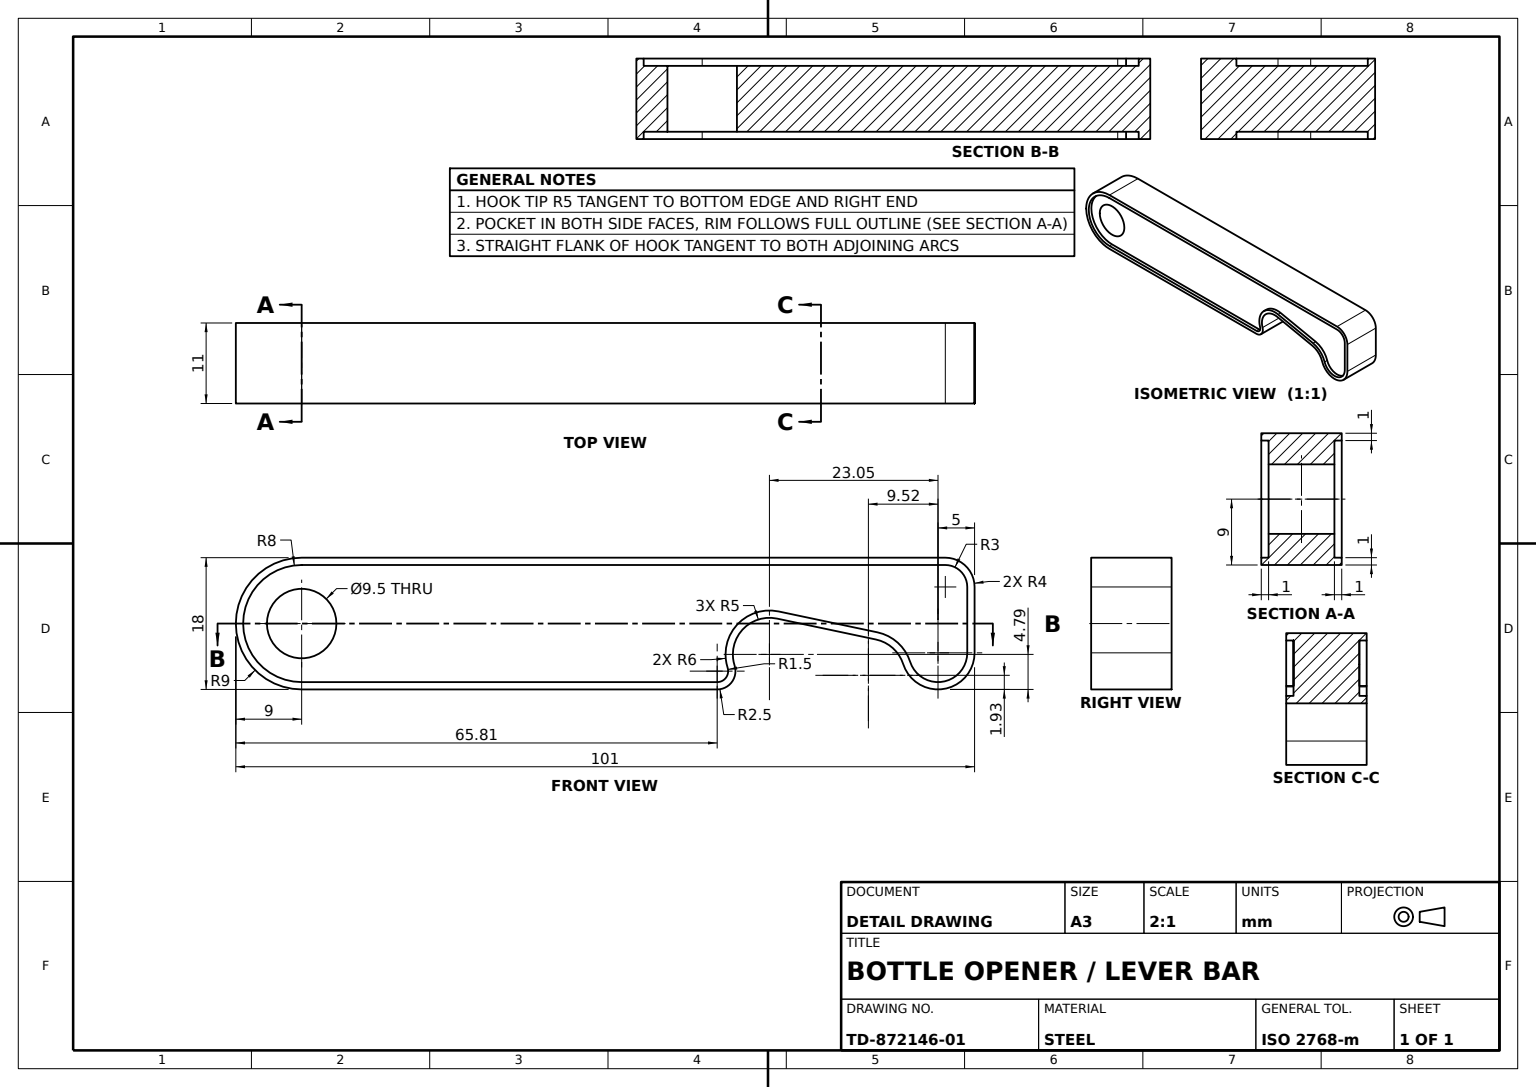
SolidWorks part; units mm, degrees
material "Plain Carbon Steel"
ref_plane "Front Plane" through (0, 0, 0) normal (0, 0, 1) x (1, 0, 0)
ref_plane "Top Plane" through (0, 0, 0) normal (0, 1, 0) x (1, 0, 0)
ref_plane "Right Plane" through (0, 0, 0) normal (1, 0, 0) x (0, 0, -1)
sketch "Hook Profile Sketch" plane through (0, 0, 0) normal (0, 0, 1) x (1, 0, 0)
  line L1 (64.9855, 0.6793) -> (78.5166, -2.179)
  line L2 (0, 9) -> (88, 9)
  line L3 (92, 5) -> (92, -4)
  line L4 (0, -9) -> (56.8094, -9)
  arc A0 (0, 9) -> (0, -9) centre (0, 0) ccw
  arc A1 (92, 5) -> (88, 9) centre (88, 5) ccw
  arc A2 (92, -4) -> (87, -9) centre (87, -4) cw
  arc A3 (82.2416, -5.5355) -> (92, -4) centre (87, -4) ccw
  arc A4 (64.9855, 0.6793) -> (59.1903, -5.7376) centre (63.9521, -4.2127) ccw
  arc A5 (82.2416, -5.5355) -> (78.5166, -2.179) centre (77.4832, -7.071) ccw
  arc A6 (59.1903, -5.7376) -> (56.8094, -9) centre (56.8094, -6.5) cw
  point P1 (-9, 0)
  dimension "D1" = 101
  dimension "D2" = 9
  dimension "D5" = 4
  dimension "D6" = 5
  dimension "D7" = 2.5
  dimension "D8" = 5
  dimension "D3" = 5
  dimension "D4" = 4
  dimension "D9" = 23.0479
  dimension "D10" = 9.2127
  dimension "D11" = 9.5168
extrude "Hook Body 9mm" add sketch "Hook Profile Sketch" along normal mid plane 9 contours A6 A4 L1 A5 A3 A2 L3 A1 L2 A0 L4
sketch "Face Rim Sketch" plane through (0, 0, 4.5) normal (0, 0, 1) x (1, 0, 0)
  line L0 (65.1922, 1.6577) -> (78.7233, -1.2006)
  line L1 (91, -4) -> (91, 5)
  line L2 (88, 8) -> (0, 8)
  line L3 (0, -8) -> (56.8094, -8)
  line L4 (64.9855, 0.6793) -> (78.5166, -2.179)
  line L5 (92, -4) -> (92, 5)
  line L6 (88, 9) -> (0, 9)
  line L7 (0, -9) -> (56.8094, -9)
  line L8 (64.9855, 0.6793) -> (78.5166, -2.179)
  line L9 (92, -4) -> (92, 5)
  line L10 (88, 9) -> (0, 9)
  line L11 (0, -9) -> (56.8094, -9)
  arc A0 (83.1933, -5.2284) -> (78.7233, -1.2006) centre (77.4832, -7.071) ccw
  arc A1 (83.1933, -5.2284) -> (91, -4) centre (87, -4) ccw
  arc A2 (91, 5) -> (88, 8) centre (88, 5) ccw
  arc A3 (0, 8) -> (0, -8) centre (0, 0) ccw
  arc A4 (56.8094, -8) -> (58.2379, -6.0425) centre (56.8094, -6.5) ccw
  arc A5 (65.1922, 1.6577) -> (58.2379, -6.0425) centre (63.9521, -4.2127) ccw
  arc A6 (56.8094, -9) -> (59.1903, -5.7376) centre (56.8094, -6.5) ccw
  arc A7 (64.9855, 0.6793) -> (59.1903, -5.7376) centre (63.9521, -4.2127) ccw
  arc A8 (82.2416, -5.5355) -> (78.5166, -2.179) centre (77.4832, -7.071) ccw
  arc A9 (82.2416, -5.5355) -> (92, -4) centre (87, -4) ccw
  arc A10 (92, 5) -> (88, 9) centre (88, 5) ccw
  arc A11 (0, 9) -> (0, -9) centre (0, 0) ccw
  arc A12 (56.8094, -9) -> (59.1903, -5.7376) centre (56.8094, -6.5) ccw
  arc A13 (64.9855, 0.6793) -> (59.1903, -5.7376) centre (63.9521, -4.2127) ccw
  arc A14 (82.2416, -5.5355) -> (78.5166, -2.179) centre (77.4832, -7.071) ccw
  arc A15 (82.2416, -5.5355) -> (92, -4) centre (87, -4) ccw
  arc A16 (92, 5) -> (88, 9) centre (88, 5) ccw
  arc A17 (0, 9) -> (0, -9) centre (0, 0) ccw
  dimension "D1" = 0
  dimension "D2" = 1
extrude "Face Rim 1mm" add sketch "Face Rim Sketch" along normal blind 1
mirror "Face Rim Mirror" about plane through (0, 0, 0) normal (0, 0, 1) of "Face Rim 1mm"
sketch "Pivot Hole Sketch" plane through (0, 0, -4.5) normal (0, 0, -1) x (-1, 0, 0)
  circle A0 centre (0, 0) radius 4.75
  dimension "D1" = 9.5
extrude "Pivot Hole Ø9.5" cut sketch "Pivot Hole Sketch" against normal blind 16
